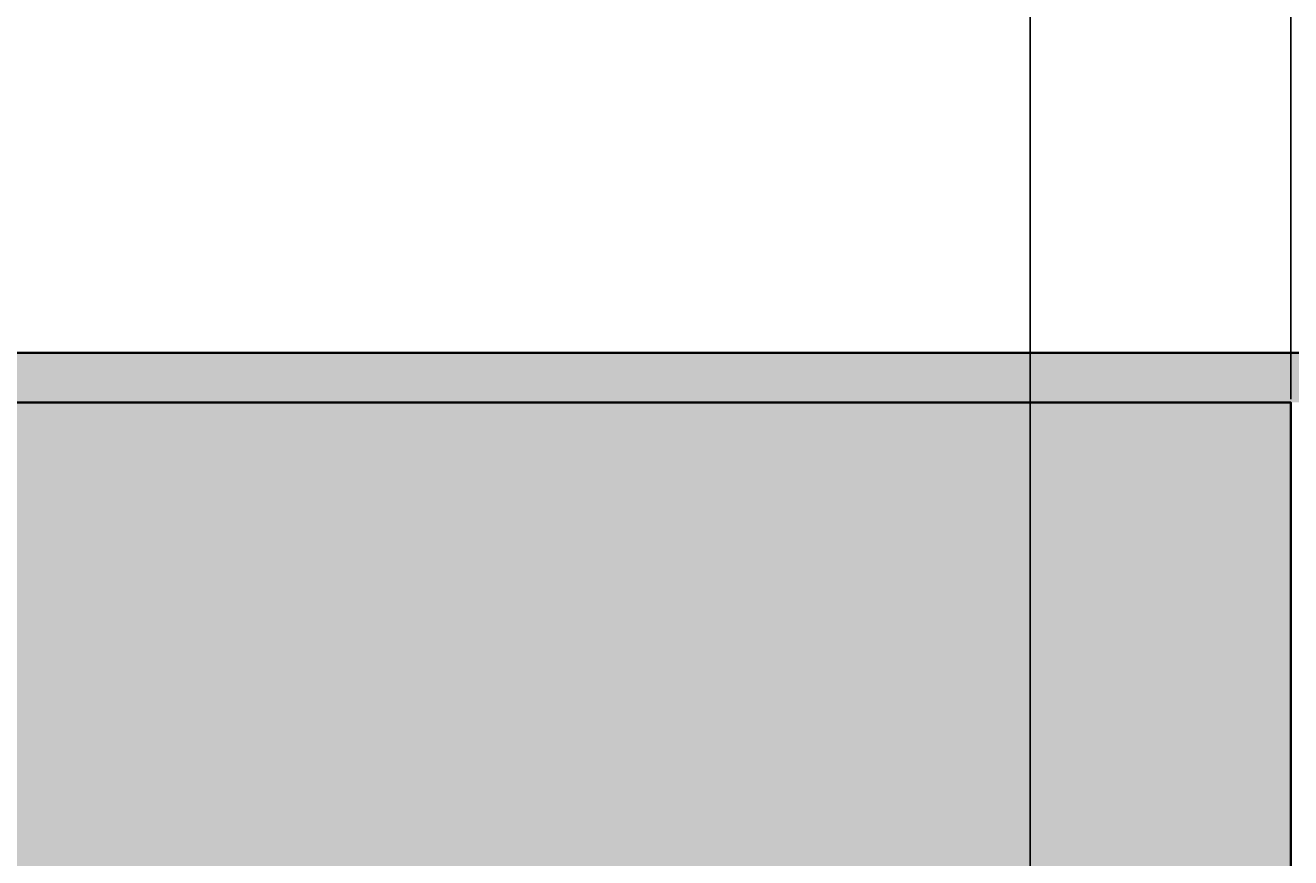
# Model space of a CAD drawing. Units: millimetres. Extents: x -11 to 280, y -4 to 208.
# Tile 52 of 55: x 211 to 237, y 156 to 173. Entities that reach past the tile are written whole.
import ezdxf

# ---------------------------------------------------------------- set-up
doc = ezdxf.new("R2010")
doc.units = ezdxf.units.MM
for name, color, linetype, lineweight in [('M-DIMS', 2, 'Continuous', 18), ('M-HYDR-EQPM', 7, 'Continuous', 35), ('M-HYDR-EQPM-PATT', 252, 'Continuous', 13)]:
    doc.layers.add(name, color=color, linetype=linetype, lineweight=lineweight)
doc.styles.get("Standard").update_dxf_attribs({"font": 'arial.ttf'})
doc.dimstyles.get("Standard").update_dxf_attribs({"dimtxt": 0.18, "dimasz": 0.18, "dimexe": 0.18, "dimexo": 0.0625, "dimgap": 0.09, "dimtad": 0, "dimtih": 1, "dimtoh": 1, "dimdec": 4, "dimzin": 0, "dimdsep": 46, "dimtxsty": 'Standard', "dimcen": 0.09, "dimadec": 0, "dimazin": 0, "dimtfac": 1, "dimtdec": 4, "dimtofl": 0, "dimtmove": 0, "dimatfit": 3, "dimfxl": 1, "dimtolj": 1, "dimtzin": 0, "dimarcsym": 0})

# ---------------------------------------------------------------- blocks, each defined once
blk = doc.blocks.new('*D5')
at = {"layer": 'Defpoints', "color": 0, "transparency": 16777216}
for p in [(24.759, 192.645), (-10.087, 11.435), (261.686, 11.435)]:
    blk.add_point(p, dxfattribs=at)
at = {"layer": 'M-DIMS', "color": 0, "lineweight": -2, "transparency": 16777216}
for p, q in [((24.696, 192.645), (-10.267, 192.645)), ((-10.087, 192.465), (-10.087, 102.222)), ((-10.087, 11.615), (-10.087, 101.858)), ((261.624, 11.435), (-10.267, 11.435))]:
    blk.add_line(p, q, dxfattribs=at)
at = {"layer": 'M-DIMS', "color": 0, "transparency": 16777216}
for points in [[(-10.117, 192.465), (-10.057, 192.465), (-10.087, 192.645)], [(-10.117, 11.615), (-10.057, 11.615), (-10.087, 11.435)]]:
    blk.add_solid(points, dxfattribs=at)
at = {"layer": 'M-DIMS', "color": 0, "transparency": 16777216, "insert": (-10.087, 102.04), "char_height": 0.18, "attachment_point": 5}
blk.add_mtext('\\A1;181.2', dxfattribs=at)
blk = doc.blocks.new('*D6')
at = {"layer": 'Defpoints', "color": 0, "transparency": 16777216}
for p in [(236.935, 207.495), (66.388, 179.241), (236.935, 165.103)]:
    blk.add_point(p, dxfattribs=at)
at = {"layer": 'M-DIMS', "color": 0, "lineweight": -2, "transparency": 16777216}
for p, q in [((66.388, 179.304), (66.388, 207.675)), ((236.935, 165.166), (236.935, 207.675)), ((66.568, 207.495), (151.206, 207.495)), ((236.755, 207.495), (152.117, 207.495))]:
    blk.add_line(p, q, dxfattribs=at)
at = {"layer": 'M-DIMS', "color": 0, "transparency": 16777216}
for points in [[(66.568, 207.525), (66.568, 207.465), (66.388, 207.495)], [(236.755, 207.525), (236.755, 207.465), (236.935, 207.495)]]:
    blk.add_solid(points, dxfattribs=at)
at = {"layer": 'M-DIMS', "color": 0, "transparency": 16777216, "insert": (151.661, 207.495), "char_height": 0.18, "attachment_point": 5}
blk.add_mtext('\\A1;170.55', dxfattribs=at)
blk = doc.blocks.new('*D20')
at = {"layer": 'Defpoints', "color": 0, "transparency": 16777216}
for p in [(231.68, 207.495), (151.022, 43.599), (231.68, 43.599)]:
    blk.add_point(p, dxfattribs=at)
at = {"layer": 'M-DIMS', "color": 0, "lineweight": -2, "transparency": 16777216}
for p, q in [((151.022, 43.662), (151.022, 207.675)), ((231.68, 43.662), (231.68, 207.675)), ((151.202, 207.495), (190.957, 207.495)), ((231.5, 207.495), (191.745, 207.495))]:
    blk.add_line(p, q, dxfattribs=at)
at = {"layer": 'M-DIMS', "color": 0, "transparency": 16777216}
for points in [[(151.202, 207.525), (151.202, 207.465), (151.022, 207.495)], [(231.5, 207.525), (231.5, 207.465), (231.68, 207.495)]]:
    blk.add_solid(points, dxfattribs=at)
at = {"layer": 'M-DIMS', "color": 0, "transparency": 16777216, "insert": (191.351, 207.495), "char_height": 0.18, "attachment_point": 5}
blk.add_mtext('\\A1;80.66', dxfattribs=at)
blk = doc.blocks.new('*D22')
at = {"layer": 'Defpoints', "color": 0, "transparency": 16777216}
for p in [(259.871, 207.495), (231.68, 34.723), (259.871, 34.723)]:
    blk.add_point(p, dxfattribs=at)
at = {"layer": 'M-DIMS', "color": 0, "lineweight": -2, "transparency": 16777216}
for p, q in [((231.68, 34.785), (231.68, 207.675)), ((259.871, 34.785), (259.871, 207.675)), ((231.86, 207.495), (245.38, 207.495)), ((259.691, 207.495), (246.171, 207.495))]:
    blk.add_line(p, q, dxfattribs=at)
at = {"layer": 'M-DIMS', "color": 0, "transparency": 16777216}
for points in [[(231.86, 207.525), (231.86, 207.465), (231.68, 207.495)], [(259.691, 207.525), (259.691, 207.465), (259.871, 207.495)]]:
    blk.add_solid(points, dxfattribs=at)
at = {"layer": 'M-DIMS', "color": 0, "transparency": 16777216, "insert": (245.776, 207.495), "char_height": 0.18, "attachment_point": 5}
blk.add_mtext('\\A1;28.19', dxfattribs=at)
blk = doc.blocks.new('*D25')
at = {"layer": 'Defpoints', "color": 0, "transparency": 16777216}
for p in [(236.935, 179.953), (205.531, 165.103), (236.935, 165.103)]:
    blk.add_point(p, dxfattribs=at)
at = {"layer": 'M-DIMS', "color": 0, "lineweight": -2, "transparency": 16777216}
for p, q in [((205.531, 165.166), (205.531, 180.133)), ((236.935, 165.166), (236.935, 180.133)), ((205.711, 179.953), (220.77, 179.953)), ((236.755, 179.953), (221.697, 179.953))]:
    blk.add_line(p, q, dxfattribs=at)
at = {"layer": 'M-DIMS', "color": 0, "transparency": 16777216}
for points in [[(205.711, 179.983), (205.711, 179.923), (205.531, 179.953)], [(236.755, 179.983), (236.755, 179.923), (236.935, 179.953)]]:
    blk.add_solid(points, dxfattribs=at)
at = {"layer": 'M-DIMS', "color": 0, "transparency": 16777216, "insert": (221.233, 179.953), "char_height": 0.18, "attachment_point": 5}
blk.add_mtext('\\A1;31.404', dxfattribs=at)

msp = doc.modelspace()

# ---------------------------------------------------------------- hatches: boundary and pattern name
at = {"layer": 'M-HYDR-EQPM-PATT'}
h = msp.add_hatch(color=256, dxfattribs=at)
h.set_gradient(color1=(248, 153, 30), color2=(248, 153, 30), tint=1)
h.paths.add_polyline_path([(236.9353, 165.103), (205.5315, 165.103), (205.5315, 144.6609), (236.9353, 144.6609)])
h.paths.add_polyline_path([(244.8074, 166.103), (205.5315, 166.103), (205.5315, 165.103), (236.9353, 165.103), (245.4299, 165.103)])
h.paths.add_polyline_path([(248.3313, 165.603, -0.4142136), (248.8313, 166.103), (245.9853, 166.103), (246.6078, 165.103), (248.8313, 165.103, -0.4142136)])
h.paths.add_polyline_path([(249.3313, 165.603, 1), (248.3313, 165.603, 0.4142136), (248.8313, 165.103, 0.4142136)])

# ---------------------------------------------------------------- linework, layer by layer
at = {"layer": 'M-HYDR-EQPM'}
msp.add_line((244.8074, 166.103), (205.5315, 166.103), dxfattribs=at)
msp.add_lwpolyline([(205.5315, 165.103), (236.9353, 165.103), (236.9353, 144.6609), (205.5315, 144.6609)], close=True, dxfattribs=at)

# ---------------------------------------------------------------- dimensions: what is measured, and where the dimension line sits
at = {"layer": 'M-DIMS'}
for base, p1, p2, override, picture, middle in [((236.9353, 207.495), (66.3875, 179.2412), (236.9353, 165.103), {"dimdec": 2, "dimlfac": 1, "dimrnd": 0, "dimzin": 0, "dimdsep": 46, "dimlunit": 2}, '*D6', (151.6614, 207.495)), ((231.6803, 207.495), (151.0217, 43.5991), (231.6803, 43.5991), {"dimdec": 2, "dimlfac": 1, "dimrnd": 0, "dimzin": 0, "dimdsep": 46, "dimlunit": 2}, '*D20', (191.351, 207.495)), ((259.871, 207.495), (231.6803, 34.7226), (259.871, 34.7226), {"dimdec": 2, "dimlfac": 1, "dimrnd": 0, "dimzin": 0, "dimdsep": 46, "dimlunit": 2}, '*D22', (245.7757, 207.495)), ((236.9353, 179.953), (205.5315, 165.103), (236.9353, 165.103), {"dimdec": 3, "dimlfac": 1, "dimrnd": 0, "dimzin": 0, "dimdsep": 46, "dimlunit": 2}, '*D25', (221.2334, 179.953))]:
    dim = msp.add_linear_dim(base=base, p1=p1, p2=p2, dimstyle='Standard', override=override, dxfattribs=at)
    dim.commit()
    dim.dimension.update_dxf_attribs({"geometry": picture, "text_midpoint": middle})
dim = msp.add_linear_dim(base=(-10.0865, 11.4346), p1=(24.7588, 192.645), p2=(261.6863, 11.4346), angle=90, dimstyle='Standard', override={"dimdec": 1, "dimlfac": 1, "dimrnd": 0, "dimzin": 0, "dimdsep": 46, "dimlunit": 2}, dxfattribs=at)
dim.commit()
dim.dimension.update_dxf_attribs({"geometry": '*D5', "text_midpoint": (-10.0865, 102.0398)})

doc.saveas('drawing.dxf')
